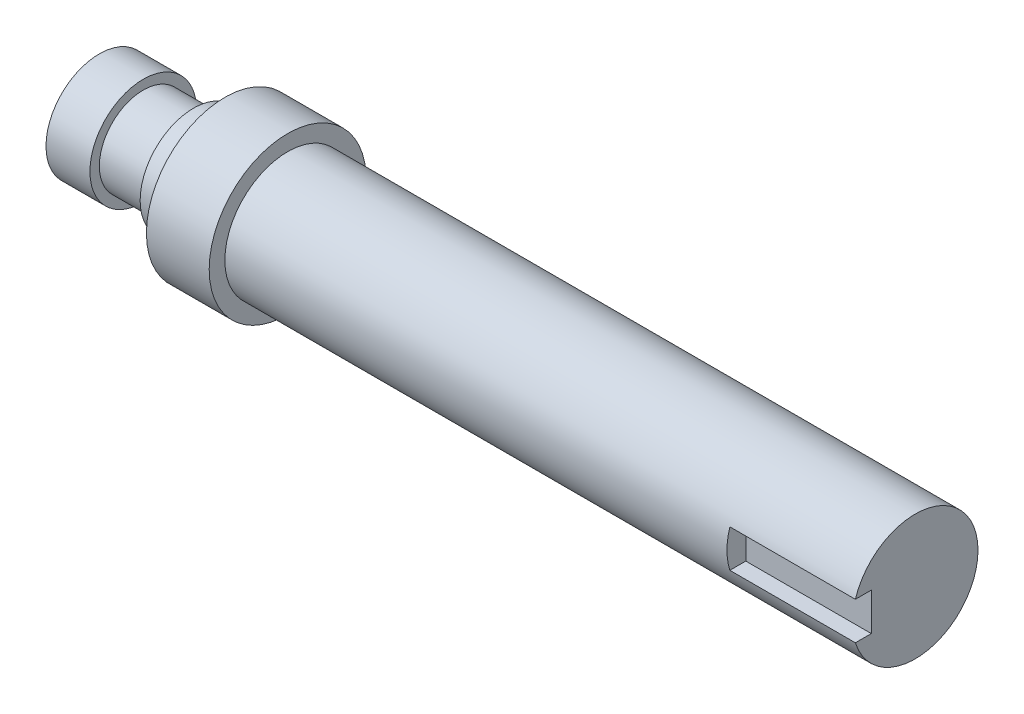
SolidWorks part; units mm, degrees
material "Plain Carbon Steel"
ref_plane "Front Plane" through (0, 0, 0) normal (0, 0, 1) x (1, 0, 0)
ref_plane "Top Plane" through (0, 0, 0) normal (0, 1, 0) x (1, 0, 0)
ref_plane "Right Plane" through (0, 0, 0) normal (1, 0, 0) x (0, 0, -1)
sketch "Shaft Profile Sketch" plane through (0, 0, 0) normal (0, 0, 1) x (1, 0, 0)
  line L0 (0, 0) -> (130, 0)
  line L1 (130, 0) -> (130, -10)
  line L2 (130, -10) -> (30, -10)
  line L3 (30, -10) -> (30, -12.5)
  line L4 (30, -12.5) -> (20, -12.5)
  line L5 (20, -8.5) -> (15, -8.5)
  line L6 (20, -12.5) -> (20, -8.5)
  line L7 (15, -7) -> (7, -7)
  line L8 (15, -8.5) -> (15, -7)
  line L9 (7, -7) -> (7, -8.5)
  line L10 (7, -8.5) -> (0, -8.5)
  line L11 (0, -8.5) -> (0, 0)
  dimension "D1" = 100
  dimension "D2" = 10
  dimension "D3" = 130
  dimension "D4" = 10
  dimension "D5" = 12.5
  dimension "D6" = 8.5
  dimension "D7" = 15
  dimension "D8" = 7
  dimension "D9" = 7
  dimension "D10" = 8.5
revolve "Stepped Shaft Body" add sketch "Shaft Profile Sketch" angle 360 about L0
ref_plane "Keyway Plane" through (0, 0, 10) normal (0, 0, 1) x (1, 0, 0)
sketch "Keyway Sketch" plane through (0, 0, 10) normal (0, 0, 1) x (1, 0, 0)
  line L0 (30, -10) -> (130, -10) construction
  line L1 (130, -10) -> (130, 10) construction
  line L2 (110, 0) -> (110, 3)
  line L3 (110, 3) -> (130, 3)
  line L4 (130, 3) -> (130, -3)
  line L5 (130, -3) -> (110, -3)
  line L6 (110, -3) -> (110, 0)
  point P10 (130, 0)
  dimension "D1" = 20
  dimension "D2" = 6
  dimension "D3" = 7
  dimension "D4" = 20
extrude "Keyway 6x20 Depth 3" cut sketch "Keyway Sketch" against normal blind 3
